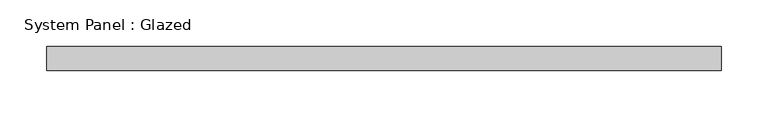
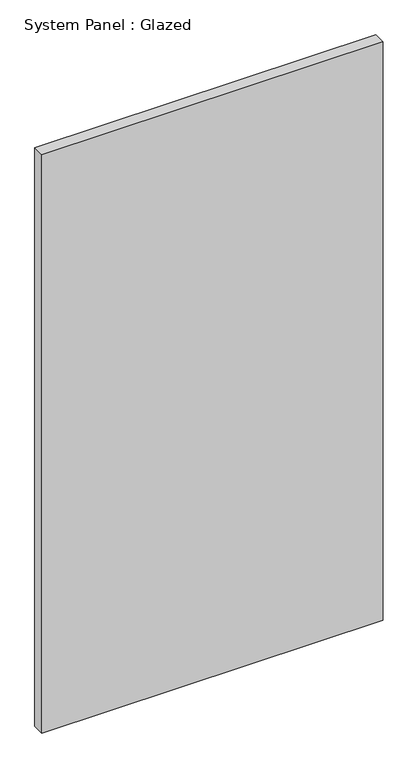
"""IFC4 building model written with IfcOpenShell, lengths in millimetres: plate geometry, System Panel : Glazed."""

from ifc_helpers import new_model, si_unit, origin, origin_with_axes, place, context, project, spatial, polyline, outline, extrude, source, transform, mapped, element, save


def system_panel_glazed_82717b58(model_context):
    return source(origin(), model_context, "Body", "SweptSolid", [
        extrude(outline(polyline([(358.775, 19.05), (-358.775, 19.05), (-358.775, 44.45), (358.775, 44.45), (358.775, 19.05)])), origin_with_axes(), (0.0, 0.0, 1.0), 1284.7908292),
    ])


if __name__ == "__main__":
    model = new_model("IFC4")
    model_context = context("Model", 3, world=origin())
    ifc_project = project(units=[si_unit("LENGTHUNIT", "METRE", prefix="MILLI")], contexts=[model_context])
    site = spatial("IfcSite", under=ifc_project)
    building = spatial("IfcBuilding", under=site)
    placement = place(None, origin())
    system_panel_glazed_shape = system_panel_glazed_82717b58(model_context)
    element("IfcPlate", 1, ObjectType="System Panel : Glazed", at=placement, inside=building, context=model_context, shape_type="MappedRepresentation", body=[
        mapped(system_panel_glazed_shape, transform((0.0, 0.0, 0.0), x_axis=(1.0, 0.0, 0.0), y_axis=(0.0, 1.0, 0.0), z_axis=(0.0, 0.0, 1.0))),
    ])
    save(model, "model.ifc")

# Revit data of these elements
# Type "System Panel : Glazed"
#   Construction Type Id = "GSP4R"
#   Analytic Construction = "1/8 in Pilkington single glazing"
#   Visual Light Transmittance = 0.9
#   Solar Heat Gain Coefficient = 0.86
#   Heat Transfer Coefficient (U) = 1.18115 BTU/(h·ft²·°F)
#   Define Thermal Properties by = 1
# Element 1 (IfcPlate, "System Panel : Glazed")
#   Materials on its faces: "Glass"
# Materials
#   "Glass": class "Glass", colour RGB 0 128 192, transparency 0.75, Description = "Soda Lime Glass", Cost = 0
